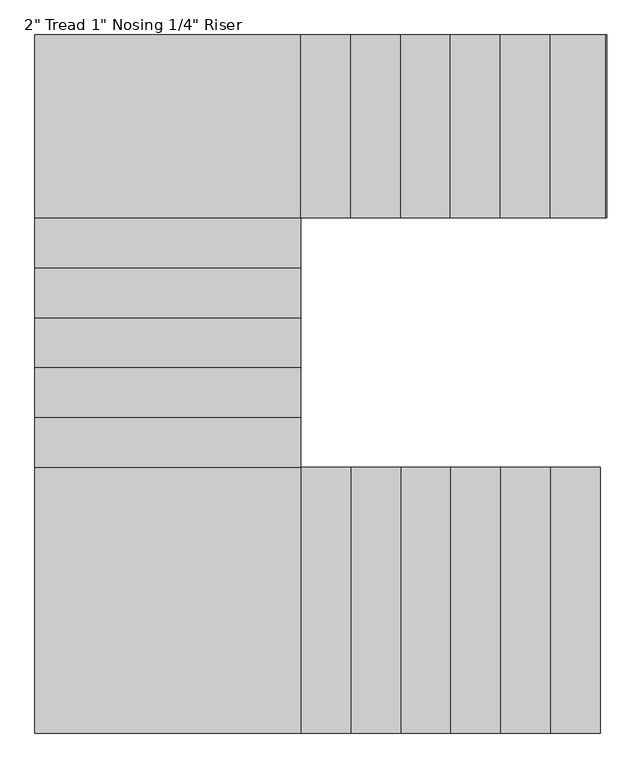
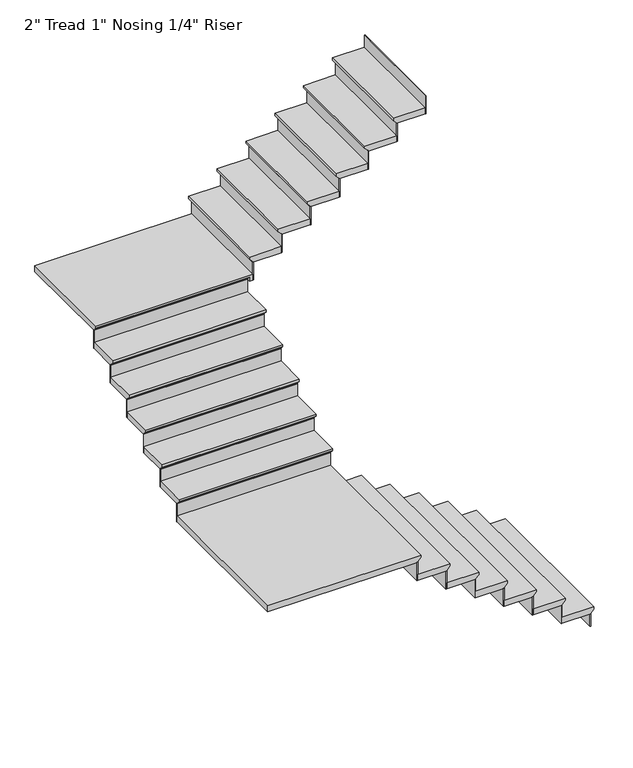
"""IFC4 building model written with IfcOpenShell, lengths in millimetres: stair flight geometry."""

from ifc_helpers import new_model, si_unit, origin, place, context, project, spatial, faceted_brep, source, transform, mapped, element, save


def stair_flight_8a4abe09(model_context):
    return source(origin(), model_context, "Body", "Brep", [
        faceted_brep([(-2515.2117403, -5163.0426559, 3181.35), (-2515.2117403, -5163.0426559, 3200.4), (-2515.2117403, -6382.2426559, 3200.4), (-2515.2117403, -6382.2426559, 3181.35), (-2540.6117403, -5163.0426559, 3155.95), (-2540.6117403, -6382.2426559, 3155.95), (-2769.2117403, -5163.0426559, 3200.4), (-2769.2117403, -6382.2426559, 3200.4), (-2540.6117403, -6382.2426559, 3149.6), (-2769.2117403, -6382.2426559, 3149.6), (-2769.2117403, -5163.0426559, 3149.6), (-2540.6117403, -5163.0426559, 3149.6)], [[[0, 1, 2, 3]], [[4, 0, 3, 5]], [[2, 1, 6, 7]], [[8, 9, 10, 11]], [[2, 7, 9, 8, 5, 3]], [[8, 11, 4, 5]], [[6, 1, 0, 4, 11, 10]], [[7, 6, 10, 9]]]),
        faceted_brep([(-2540.6117403, -5163.0426559, 3149.6), (-2540.6117403, -5163.0426559, 3048.0), (-2546.9617403, -5163.0426559, 3048.0), (-2546.9617403, -5163.0426559, 3149.6), (-2540.6117403, -6382.2426559, 3149.6), (-2546.9617403, -6382.2426559, 3149.6), (-2546.9617403, -6382.2426559, 3048.0), (-2540.6117403, -6382.2426559, 3048.0)], [[[0, 1, 2, 3]], [[4, 5, 6, 7]], [[1, 0, 4, 7]], [[2, 1, 7, 6]], [[3, 2, 6, 5]], [[0, 3, 5, 4]]]),
        faceted_brep([(-2769.2117403, -5163.0426559, 3302.0), (-2769.2117403, -5163.0426559, 3149.6), (-2775.5617403, -5163.0426559, 3149.6), (-2775.5617403, -5163.0426559, 3302.0), (-2769.2117403, -6382.2426559, 3302.0), (-2775.5617403, -6382.2426559, 3302.0), (-2775.5617403, -6382.2426559, 3149.6), (-2769.2117403, -6382.2426559, 3149.6)], [[[0, 1, 2, 3]], [[4, 5, 6, 7]], [[1, 0, 4, 7]], [[2, 1, 7, 6]], [[3, 2, 6, 5]], [[0, 3, 5, 4]]]),
        faceted_brep([(-2743.8117403, -6382.2426559, 3352.8), (-2743.8117403, -5163.0426559, 3352.8), (-2997.8117403, -5163.0426559, 3352.8), (-2997.8117403, -6382.2426559, 3352.8), (-2769.2117403, -6382.2426559, 3302.0), (-2997.8117403, -6382.2426559, 3302.0), (-2997.8117403, -5163.0426559, 3302.0), (-2769.2117403, -5163.0426559, 3302.0), (-2769.2117403, -6382.2426559, 3308.35), (-2743.8117403, -6382.2426559, 3333.75), (-2769.2117403, -5163.0426559, 3308.35), (-2743.8117403, -5163.0426559, 3333.75)], [[[0, 1, 2, 3]], [[4, 5, 6, 7]], [[0, 3, 5, 4, 8, 9]], [[4, 7, 10, 8]], [[2, 1, 11, 10, 7, 6]], [[3, 2, 6, 5]], [[11, 1, 0, 9]], [[10, 11, 9, 8]]]),
        faceted_brep([(-2997.8117403, -5163.0426559, 3454.4), (-2997.8117403, -5163.0426559, 3302.0), (-3004.1617403, -5163.0426559, 3302.0), (-3004.1617403, -5163.0426559, 3454.4), (-2997.8117403, -6382.2426559, 3454.4), (-3004.1617403, -6382.2426559, 3454.4), (-3004.1617403, -6382.2426559, 3302.0), (-2997.8117403, -6382.2426559, 3302.0)], [[[0, 1, 2, 3]], [[4, 5, 6, 7]], [[1, 0, 4, 7]], [[2, 1, 7, 6]], [[3, 2, 6, 5]], [[0, 3, 5, 4]]]),
        faceted_brep([(-2972.4117403, -6382.2426559, 3505.2), (-2972.4117403, -5163.0426559, 3505.2), (-3226.4117403, -5163.0426559, 3505.2), (-3226.4117403, -6382.2426559, 3505.2), (-2997.8117403, -6382.2426559, 3454.4), (-3226.4117403, -6382.2426559, 3454.4), (-3226.4117403, -5163.0426559, 3454.4), (-2997.8117403, -5163.0426559, 3454.4), (-2997.8117403, -6382.2426559, 3460.75), (-2972.4117403, -6382.2426559, 3486.15), (-2997.8117403, -5163.0426559, 3460.75), (-2972.4117403, -5163.0426559, 3486.15)], [[[0, 1, 2, 3]], [[4, 5, 6, 7]], [[0, 3, 5, 4, 8, 9]], [[4, 7, 10, 8]], [[2, 1, 11, 10, 7, 6]], [[3, 2, 6, 5]], [[11, 1, 0, 9]], [[10, 11, 9, 8]]]),
        faceted_brep([(-3226.4117403, -5163.0426559, 3606.8), (-3226.4117403, -5163.0426559, 3454.4), (-3232.7617403, -5163.0426559, 3454.4), (-3232.7617403, -5163.0426559, 3606.8), (-3226.4117403, -6382.2426559, 3606.8), (-3232.7617403, -6382.2426559, 3606.8), (-3232.7617403, -6382.2426559, 3454.4), (-3226.4117403, -6382.2426559, 3454.4)], [[[0, 1, 2, 3]], [[4, 5, 6, 7]], [[1, 0, 4, 7]], [[2, 1, 7, 6]], [[3, 2, 6, 5]], [[0, 3, 5, 4]]]),
        faceted_brep([(-3201.0117403, -6382.2426559, 3657.6), (-3201.0117403, -5163.0426559, 3657.6), (-3455.0117403, -5163.0426559, 3657.6), (-3455.0117403, -6382.2426559, 3657.6), (-3226.4117403, -6382.2426559, 3606.8), (-3455.0117403, -6382.2426559, 3606.8), (-3455.0117403, -5163.0426559, 3606.8), (-3226.4117403, -5163.0426559, 3606.8), (-3226.4117403, -6382.2426559, 3613.15), (-3201.0117403, -6382.2426559, 3638.55), (-3226.4117403, -5163.0426559, 3613.15), (-3201.0117403, -5163.0426559, 3638.55)], [[[0, 1, 2, 3]], [[4, 5, 6, 7]], [[0, 3, 5, 4, 8, 9]], [[4, 7, 10, 8]], [[2, 1, 11, 10, 7, 6]], [[3, 2, 6, 5]], [[11, 1, 0, 9]], [[10, 11, 9, 8]]]),
        faceted_brep([(-3455.0117403, -5163.0426559, 3759.2), (-3455.0117403, -5163.0426559, 3606.8), (-3461.3617403, -5163.0426559, 3606.8), (-3461.3617403, -5163.0426559, 3759.2), (-3455.0117403, -6382.2426559, 3759.2), (-3461.3617403, -6382.2426559, 3759.2), (-3461.3617403, -6382.2426559, 3606.8), (-3455.0117403, -6382.2426559, 3606.8)], [[[0, 1, 2, 3]], [[4, 5, 6, 7]], [[1, 0, 4, 7]], [[2, 1, 7, 6]], [[3, 2, 6, 5]], [[0, 3, 5, 4]]]),
        faceted_brep([(-3429.6117403, -6382.2426559, 3810.0), (-3429.6117403, -5163.0426559, 3810.0), (-3683.6117403, -5163.0426559, 3810.0), (-3683.6117403, -6382.2426559, 3810.0), (-3455.0117403, -6382.2426559, 3759.2), (-3683.6117403, -6382.2426559, 3759.2), (-3683.6117403, -5163.0426559, 3759.2), (-3455.0117403, -5163.0426559, 3759.2), (-3455.0117403, -6382.2426559, 3765.55), (-3429.6117403, -6382.2426559, 3790.95), (-3455.0117403, -5163.0426559, 3765.55), (-3429.6117403, -5163.0426559, 3790.95)], [[[0, 1, 2, 3]], [[4, 5, 6, 7]], [[0, 3, 5, 4, 8, 9]], [[4, 7, 10, 8]], [[2, 1, 11, 10, 7, 6]], [[3, 2, 6, 5]], [[11, 1, 0, 9]], [[10, 11, 9, 8]]]),
        faceted_brep([(-3683.6117403, -5163.0426559, 3911.6), (-3683.6117403, -5163.0426559, 3759.2), (-3689.9617403, -5163.0426559, 3759.2), (-3689.9617403, -5163.0426559, 3911.6), (-3683.6117403, -6382.2426559, 3911.6), (-3689.9617403, -6382.2426559, 3911.6), (-3689.9617403, -6382.2426559, 3759.2), (-3683.6117403, -6382.2426559, 3759.2)], [[[0, 1, 2, 3]], [[4, 5, 6, 7]], [[1, 0, 4, 7]], [[2, 1, 7, 6]], [[3, 2, 6, 5]], [[0, 3, 5, 4]]]),
        faceted_brep([(-3658.2117403, -6382.2426559, 3962.4), (-3658.2117403, -5163.0426559, 3962.4), (-3912.2117403, -5163.0426559, 3962.4), (-3912.2117403, -6382.2426559, 3962.4), (-3683.6117403, -6382.2426559, 3911.6), (-3912.2117403, -6382.2426559, 3911.6), (-3912.2117403, -5163.0426559, 3911.6), (-3683.6117403, -5163.0426559, 3911.6), (-3683.6117403, -6382.2426559, 3917.95), (-3658.2117403, -6382.2426559, 3943.35), (-3683.6117403, -5163.0426559, 3917.95), (-3658.2117403, -5163.0426559, 3943.35)], [[[0, 1, 2, 3]], [[4, 5, 6, 7]], [[0, 3, 5, 4, 8, 9]], [[4, 7, 10, 8]], [[2, 1, 11, 10, 7, 6]], [[3, 2, 6, 5]], [[11, 1, 0, 9]], [[10, 11, 9, 8]]]),
        faceted_brep([(-3912.2117403, -5163.0426559, 4064.0), (-3912.2117403, -5163.0426559, 3911.6), (-3918.5617403, -5163.0426559, 3911.6), (-3918.5617403, -5163.0426559, 4064.0), (-3912.2117403, -6382.2426559, 4064.0), (-3918.5617403, -6382.2426559, 4064.0), (-3918.5617403, -6382.2426559, 3911.6), (-3912.2117403, -6382.2426559, 3911.6)], [[[0, 1, 2, 3]], [[4, 5, 6, 7]], [[1, 0, 4, 7]], [[2, 1, 7, 6]], [[3, 2, 6, 5]], [[0, 3, 5, 4]]]),
        faceted_brep([(-5106.0117403, -5137.6426559, 4114.8), (-5106.0117403, -6382.2426559, 4114.8), (-3886.8117403, -6382.2426559, 4114.8), (-3886.8117403, -5137.6426559, 4114.8), (-5106.0117403, -6382.2426559, 4064.0), (-5106.0117403, -5137.6426559, 4064.0), (-3886.8117403, -5137.6426559, 4064.0), (-3886.8117403, -5163.0426559, 4064.0), (-3912.2117403, -5163.0426559, 4064.0), (-3912.2117403, -6382.2426559, 4064.0), (-3912.2117403, -6382.2426559, 4070.35), (-3886.8117403, -6382.2426559, 4095.75), (-3912.2117403, -5163.0426559, 4070.35), (-3886.8117403, -5163.0426559, 4095.75)], [[[0, 1, 2, 3]], [[4, 5, 6, 7, 8, 9]], [[1, 0, 5, 4]], [[2, 1, 4, 9, 10, 11]], [[9, 8, 12, 10]], [[8, 7, 13, 12]], [[3, 2, 11, 13, 7, 6]], [[0, 3, 6, 5]], [[11, 10, 12, 13]]]),
        faceted_brep([(-3886.8117403, -5137.6426559, 4216.4), (-3886.8117403, -5137.6426559, 4064.0), (-3886.8117403, -5131.2926559, 4064.0), (-3886.8117403, -5131.2926559, 4216.4), (-5106.0117403, -5137.6426559, 4216.4), (-5106.0117403, -5131.2926559, 4216.4), (-5106.0117403, -5131.2926559, 4064.0), (-5106.0117403, -5137.6426559, 4064.0)], [[[0, 1, 2, 3]], [[4, 5, 6, 7]], [[1, 0, 4, 7]], [[2, 1, 7, 6]], [[3, 2, 6, 5]], [[0, 3, 5, 4]]]),
        faceted_brep([(-5106.0117403, -5163.0426559, 4267.2), (-3886.8117403, -5163.0426559, 4267.2), (-3886.8117403, -4909.0426559, 4267.2), (-5106.0117403, -4909.0426559, 4267.2), (-5106.0117403, -5137.6426559, 4216.4), (-5106.0117403, -4909.0426559, 4216.4), (-3886.8117403, -4909.0426559, 4216.4), (-3886.8117403, -5137.6426559, 4216.4), (-5106.0117403, -5137.6426559, 4222.75), (-5106.0117403, -5163.0426559, 4248.15), (-3886.8117403, -5137.6426559, 4222.75), (-3886.8117403, -5163.0426559, 4248.15)], [[[0, 1, 2, 3]], [[4, 5, 6, 7]], [[0, 3, 5, 4, 8, 9]], [[4, 7, 10, 8]], [[2, 1, 11, 10, 7, 6]], [[3, 2, 6, 5]], [[11, 1, 0, 9]], [[10, 11, 9, 8]]]),
        faceted_brep([(-3886.8117403, -4909.0426559, 4368.8), (-3886.8117403, -4909.0426559, 4216.4), (-3886.8117403, -4902.6926559, 4216.4), (-3886.8117403, -4902.6926559, 4368.8), (-5106.0117403, -4909.0426559, 4368.8), (-5106.0117403, -4902.6926559, 4368.8), (-5106.0117403, -4902.6926559, 4216.4), (-5106.0117403, -4909.0426559, 4216.4)], [[[0, 1, 2, 3]], [[4, 5, 6, 7]], [[1, 0, 4, 7]], [[2, 1, 7, 6]], [[3, 2, 6, 5]], [[0, 3, 5, 4]]]),
        faceted_brep([(-5106.0117403, -4934.4426559, 4419.6), (-3886.8117403, -4934.4426559, 4419.6), (-3886.8117403, -4680.4426559, 4419.6), (-5106.0117403, -4680.4426559, 4419.6), (-5106.0117403, -4909.0426559, 4368.8), (-5106.0117403, -4680.4426559, 4368.8), (-3886.8117403, -4680.4426559, 4368.8), (-3886.8117403, -4909.0426559, 4368.8), (-5106.0117403, -4909.0426559, 4375.15), (-5106.0117403, -4934.4426559, 4400.55), (-3886.8117403, -4909.0426559, 4375.15), (-3886.8117403, -4934.4426559, 4400.55)], [[[0, 1, 2, 3]], [[4, 5, 6, 7]], [[0, 3, 5, 4, 8, 9]], [[4, 7, 10, 8]], [[2, 1, 11, 10, 7, 6]], [[3, 2, 6, 5]], [[11, 1, 0, 9]], [[10, 11, 9, 8]]]),
        faceted_brep([(-3886.8117403, -4680.4426559, 4521.2), (-3886.8117403, -4680.4426559, 4368.8), (-3886.8117403, -4674.0926559, 4368.8), (-3886.8117403, -4674.0926559, 4521.2), (-5106.0117403, -4680.4426559, 4521.2), (-5106.0117403, -4674.0926559, 4521.2), (-5106.0117403, -4674.0926559, 4368.8), (-5106.0117403, -4680.4426559, 4368.8)], [[[0, 1, 2, 3]], [[4, 5, 6, 7]], [[1, 0, 4, 7]], [[2, 1, 7, 6]], [[3, 2, 6, 5]], [[0, 3, 5, 4]]]),
        faceted_brep([(-5106.0117403, -4705.8426559, 4572.0), (-3886.8117403, -4705.8426559, 4572.0), (-3886.8117403, -4451.8426559, 4572.0), (-5106.0117403, -4451.8426559, 4572.0), (-5106.0117403, -4680.4426559, 4521.2), (-5106.0117403, -4451.8426559, 4521.2), (-3886.8117403, -4451.8426559, 4521.2), (-3886.8117403, -4680.4426559, 4521.2), (-5106.0117403, -4680.4426559, 4527.55), (-5106.0117403, -4705.8426559, 4552.95), (-3886.8117403, -4680.4426559, 4527.55), (-3886.8117403, -4705.8426559, 4552.95)], [[[0, 1, 2, 3]], [[4, 5, 6, 7]], [[0, 3, 5, 4, 8, 9]], [[4, 7, 10, 8]], [[2, 1, 11, 10, 7, 6]], [[3, 2, 6, 5]], [[11, 1, 0, 9]], [[10, 11, 9, 8]]]),
        faceted_brep([(-3886.8117403, -4451.8426559, 4673.6), (-3886.8117403, -4451.8426559, 4521.2), (-3886.8117403, -4445.4926559, 4521.2), (-3886.8117403, -4445.4926559, 4673.6), (-5106.0117403, -4451.8426559, 4673.6), (-5106.0117403, -4445.4926559, 4673.6), (-5106.0117403, -4445.4926559, 4521.2), (-5106.0117403, -4451.8426559, 4521.2)], [[[0, 1, 2, 3]], [[4, 5, 6, 7]], [[1, 0, 4, 7]], [[2, 1, 7, 6]], [[3, 2, 6, 5]], [[0, 3, 5, 4]]]),
        faceted_brep([(-5106.0117403, -4477.2426559, 4724.4), (-3886.8117403, -4477.2426559, 4724.4), (-3886.8117403, -4223.2426559, 4724.4), (-5106.0117403, -4223.2426559, 4724.4), (-5106.0117403, -4451.8426559, 4673.6), (-5106.0117403, -4223.2426559, 4673.6), (-3886.8117403, -4223.2426559, 4673.6), (-3886.8117403, -4451.8426559, 4673.6), (-5106.0117403, -4451.8426559, 4679.95), (-5106.0117403, -4477.2426559, 4705.35), (-3886.8117403, -4451.8426559, 4679.95), (-3886.8117403, -4477.2426559, 4705.35)], [[[0, 1, 2, 3]], [[4, 5, 6, 7]], [[0, 3, 5, 4, 8, 9]], [[4, 7, 10, 8]], [[2, 1, 11, 10, 7, 6]], [[3, 2, 6, 5]], [[11, 1, 0, 9]], [[10, 11, 9, 8]]]),
        faceted_brep([(-3886.8117403, -4223.2426559, 4826.0), (-3886.8117403, -4223.2426559, 4673.6), (-3886.8117403, -4216.8926559, 4673.6), (-3886.8117403, -4216.8926559, 4826.0), (-5106.0117403, -4223.2426559, 4826.0), (-5106.0117403, -4216.8926559, 4826.0), (-5106.0117403, -4216.8926559, 4673.6), (-5106.0117403, -4223.2426559, 4673.6)], [[[0, 1, 2, 3]], [[4, 5, 6, 7]], [[1, 0, 4, 7]], [[2, 1, 7, 6]], [[3, 2, 6, 5]], [[0, 3, 5, 4]]]),
        faceted_brep([(-5106.0117403, -4248.6426559, 4876.8), (-3886.8117403, -4248.6426559, 4876.8), (-3886.8117403, -3994.6426559, 4876.8), (-5106.0117403, -3994.6426559, 4876.8), (-5106.0117403, -4223.2426559, 4826.0), (-5106.0117403, -3994.6426559, 4826.0), (-3886.8117403, -3994.6426559, 4826.0), (-3886.8117403, -4223.2426559, 4826.0), (-5106.0117403, -4223.2426559, 4832.35), (-5106.0117403, -4248.6426559, 4857.75), (-3886.8117403, -4223.2426559, 4832.35), (-3886.8117403, -4248.6426559, 4857.75)], [[[0, 1, 2, 3]], [[4, 5, 6, 7]], [[0, 3, 5, 4, 8, 9]], [[4, 7, 10, 8]], [[2, 1, 11, 10, 7, 6]], [[3, 2, 6, 5]], [[11, 1, 0, 9]], [[10, 11, 9, 8]]]),
        faceted_brep([(-3886.8117403, -3994.6426559, 4978.4), (-3886.8117403, -3994.6426559, 4826.0), (-3886.8117403, -3988.2926559, 4826.0), (-3886.8117403, -3988.2926559, 4978.4), (-5106.0117403, -3994.6426559, 4978.4), (-5106.0117403, -3988.2926559, 4978.4), (-5106.0117403, -3988.2926559, 4826.0), (-5106.0117403, -3994.6426559, 4826.0)], [[[0, 1, 2, 3]], [[4, 5, 6, 7]], [[1, 0, 4, 7]], [[2, 1, 7, 6]], [[3, 2, 6, 5]], [[0, 3, 5, 4]]]),
        faceted_brep([(-3861.4117403, -3181.8426559, 5029.2), (-5106.0117403, -3181.8426559, 5029.2), (-5106.0117403, -4020.0426559, 5029.2), (-3861.4117403, -4020.0426559, 5029.2), (-5106.0117403, -3181.8426559, 4978.4), (-3861.4117403, -3181.8426559, 4978.4), (-3861.4117403, -4020.0426559, 4978.4), (-3886.8117403, -4020.0426559, 4978.4), (-3886.8117403, -3994.6426559, 4978.4), (-5106.0117403, -3994.6426559, 4978.4), (-5106.0117403, -3994.6426559, 4984.75), (-5106.0117403, -4020.0426559, 5010.15), (-3886.8117403, -3994.6426559, 4984.75), (-3886.8117403, -4020.0426559, 5010.15)], [[[0, 1, 2, 3]], [[4, 5, 6, 7, 8, 9]], [[1, 0, 5, 4]], [[2, 1, 4, 9, 10, 11]], [[9, 8, 12, 10]], [[8, 7, 13, 12]], [[3, 2, 11, 13, 7, 6]], [[0, 3, 6, 5]], [[11, 10, 12, 13]]]),
        faceted_brep([(-3861.4117403, -4020.0426559, 5130.8), (-3861.4117403, -4020.0426559, 4978.4), (-3855.0617403, -4020.0426559, 4978.4), (-3855.0617403, -4020.0426559, 5130.8), (-3861.4117403, -3181.8426559, 5130.8), (-3855.0617403, -3181.8426559, 5130.8), (-3855.0617403, -3181.8426559, 4978.4), (-3861.4117403, -3181.8426559, 4978.4)], [[[0, 1, 2, 3]], [[4, 5, 6, 7]], [[1, 0, 4, 7]], [[2, 1, 7, 6]], [[3, 2, 6, 5]], [[0, 3, 5, 4]]]),
        faceted_brep([(-3886.8117403, -3181.8426559, 5181.6), (-3886.8117403, -4020.0426559, 5181.6), (-3632.8117403, -4020.0426559, 5181.6), (-3632.8117403, -3181.8426559, 5181.6), (-3861.4117403, -3181.8426559, 5130.8), (-3632.8117403, -3181.8426559, 5130.8), (-3632.8117403, -4020.0426559, 5130.8), (-3861.4117403, -4020.0426559, 5130.8), (-3861.4117403, -3181.8426559, 5137.15), (-3886.8117403, -3181.8426559, 5162.55), (-3861.4117403, -4020.0426559, 5137.15), (-3886.8117403, -4020.0426559, 5162.55)], [[[0, 1, 2, 3]], [[4, 5, 6, 7]], [[0, 3, 5, 4, 8, 9]], [[4, 7, 10, 8]], [[2, 1, 11, 10, 7, 6]], [[3, 2, 6, 5]], [[11, 1, 0, 9]], [[10, 11, 9, 8]]]),
        faceted_brep([(-3632.8117403, -4020.0426559, 5283.2), (-3632.8117403, -4020.0426559, 5130.8), (-3626.4617403, -4020.0426559, 5130.8), (-3626.4617403, -4020.0426559, 5283.2), (-3632.8117403, -3181.8426559, 5283.2), (-3626.4617403, -3181.8426559, 5283.2), (-3626.4617403, -3181.8426559, 5130.8), (-3632.8117403, -3181.8426559, 5130.8)], [[[0, 1, 2, 3]], [[4, 5, 6, 7]], [[1, 0, 4, 7]], [[2, 1, 7, 6]], [[3, 2, 6, 5]], [[0, 3, 5, 4]]]),
        faceted_brep([(-3658.2117403, -3181.8426559, 5334.0), (-3658.2117403, -4020.0426559, 5334.0), (-3404.2117403, -4020.0426559, 5334.0), (-3404.2117403, -3181.8426559, 5334.0), (-3632.8117403, -3181.8426559, 5283.2), (-3404.2117403, -3181.8426559, 5283.2), (-3404.2117403, -4020.0426559, 5283.2), (-3632.8117403, -4020.0426559, 5283.2), (-3632.8117403, -3181.8426559, 5289.55), (-3658.2117403, -3181.8426559, 5314.95), (-3632.8117403, -4020.0426559, 5289.55), (-3658.2117403, -4020.0426559, 5314.95)], [[[0, 1, 2, 3]], [[4, 5, 6, 7]], [[0, 3, 5, 4, 8, 9]], [[4, 7, 10, 8]], [[2, 1, 11, 10, 7, 6]], [[3, 2, 6, 5]], [[11, 1, 0, 9]], [[10, 11, 9, 8]]]),
        faceted_brep([(-3404.2117403, -4020.0426559, 5435.6), (-3404.2117403, -4020.0426559, 5283.2), (-3397.8617403, -4020.0426559, 5283.2), (-3397.8617403, -4020.0426559, 5435.6), (-3404.2117403, -3181.8426559, 5435.6), (-3397.8617403, -3181.8426559, 5435.6), (-3397.8617403, -3181.8426559, 5283.2), (-3404.2117403, -3181.8426559, 5283.2)], [[[0, 1, 2, 3]], [[4, 5, 6, 7]], [[1, 0, 4, 7]], [[2, 1, 7, 6]], [[3, 2, 6, 5]], [[0, 3, 5, 4]]]),
        faceted_brep([(-3429.6117403, -3181.8426559, 5486.4), (-3429.6117403, -4020.0426559, 5486.4), (-3175.6117403, -4020.0426559, 5486.4), (-3175.6117403, -3181.8426559, 5486.4), (-3404.2117403, -3181.8426559, 5435.6), (-3175.6117403, -3181.8426559, 5435.6), (-3175.6117403, -4020.0426559, 5435.6), (-3404.2117403, -4020.0426559, 5435.6), (-3404.2117403, -3181.8426559, 5441.95), (-3429.6117403, -3181.8426559, 5467.35), (-3404.2117403, -4020.0426559, 5441.95), (-3429.6117403, -4020.0426559, 5467.35)], [[[0, 1, 2, 3]], [[4, 5, 6, 7]], [[0, 3, 5, 4, 8, 9]], [[4, 7, 10, 8]], [[2, 1, 11, 10, 7, 6]], [[3, 2, 6, 5]], [[11, 1, 0, 9]], [[10, 11, 9, 8]]]),
        faceted_brep([(-3175.6117403, -4020.0426559, 5588.0), (-3175.6117403, -4020.0426559, 5435.6), (-3169.2617403, -4020.0426559, 5435.6), (-3169.2617403, -4020.0426559, 5588.0), (-3175.6117403, -3181.8426559, 5588.0), (-3169.2617403, -3181.8426559, 5588.0), (-3169.2617403, -3181.8426559, 5435.6), (-3175.6117403, -3181.8426559, 5435.6)], [[[0, 1, 2, 3]], [[4, 5, 6, 7]], [[1, 0, 4, 7]], [[2, 1, 7, 6]], [[3, 2, 6, 5]], [[0, 3, 5, 4]]]),
        faceted_brep([(-3201.0117403, -3181.8426559, 5638.8), (-3201.0117403, -4020.0426559, 5638.8), (-2947.0117403, -4020.0426559, 5638.8), (-2947.0117403, -3181.8426559, 5638.8), (-3175.6117403, -3181.8426559, 5588.0), (-2947.0117403, -3181.8426559, 5588.0), (-2947.0117403, -4020.0426559, 5588.0), (-3175.6117403, -4020.0426559, 5588.0), (-3175.6117403, -3181.8426559, 5594.35), (-3201.0117403, -3181.8426559, 5619.75), (-3175.6117403, -4020.0426559, 5594.35), (-3201.0117403, -4020.0426559, 5619.75)], [[[0, 1, 2, 3]], [[4, 5, 6, 7]], [[0, 3, 5, 4, 8, 9]], [[4, 7, 10, 8]], [[2, 1, 11, 10, 7, 6]], [[3, 2, 6, 5]], [[11, 1, 0, 9]], [[10, 11, 9, 8]]]),
        faceted_brep([(-2947.0117403, -4020.0426559, 5740.4), (-2947.0117403, -4020.0426559, 5588.0), (-2940.6617403, -4020.0426559, 5588.0), (-2940.6617403, -4020.0426559, 5740.4), (-2947.0117403, -3181.8426559, 5740.4), (-2940.6617403, -3181.8426559, 5740.4), (-2940.6617403, -3181.8426559, 5588.0), (-2947.0117403, -3181.8426559, 5588.0)], [[[0, 1, 2, 3]], [[4, 5, 6, 7]], [[1, 0, 4, 7]], [[2, 1, 7, 6]], [[3, 2, 6, 5]], [[0, 3, 5, 4]]]),
        faceted_brep([(-2972.4117403, -3181.8426559, 5791.2), (-2972.4117403, -4020.0426559, 5791.2), (-2718.4117403, -4020.0426559, 5791.2), (-2718.4117403, -3181.8426559, 5791.2), (-2947.0117403, -3181.8426559, 5740.4), (-2718.4117403, -3181.8426559, 5740.4), (-2718.4117403, -4020.0426559, 5740.4), (-2947.0117403, -4020.0426559, 5740.4), (-2947.0117403, -3181.8426559, 5746.75), (-2972.4117403, -3181.8426559, 5772.15), (-2947.0117403, -4020.0426559, 5746.75), (-2972.4117403, -4020.0426559, 5772.15)], [[[0, 1, 2, 3]], [[4, 5, 6, 7]], [[0, 3, 5, 4, 8, 9]], [[4, 7, 10, 8]], [[2, 1, 11, 10, 7, 6]], [[3, 2, 6, 5]], [[11, 1, 0, 9]], [[10, 11, 9, 8]]]),
        faceted_brep([(-2718.4117403, -4020.0426559, 5892.8), (-2718.4117403, -4020.0426559, 5740.4), (-2712.0617403, -4020.0426559, 5740.4), (-2712.0617403, -4020.0426559, 5892.8), (-2718.4117403, -3181.8426559, 5892.8), (-2712.0617403, -3181.8426559, 5892.8), (-2712.0617403, -3181.8426559, 5740.4), (-2718.4117403, -3181.8426559, 5740.4)], [[[0, 1, 2, 3]], [[4, 5, 6, 7]], [[1, 0, 4, 7]], [[2, 1, 7, 6]], [[3, 2, 6, 5]], [[0, 3, 5, 4]]]),
        faceted_brep([(-2489.8117403, -4020.0426559, 6045.2), (-2489.8117403, -4020.0426559, 5892.8), (-2483.4617403, -4020.0426559, 5892.8), (-2483.4617403, -4020.0426559, 6045.2), (-2489.8117403, -3181.8426559, 6045.2), (-2483.4617403, -3181.8426559, 6045.2), (-2483.4617403, -3181.8426559, 5892.8), (-2489.8117403, -3181.8426559, 5892.8)], [[[0, 1, 2, 3]], [[4, 5, 6, 7]], [[1, 0, 4, 7]], [[2, 1, 7, 6]], [[3, 2, 6, 5]], [[0, 3, 5, 4]]]),
        faceted_brep([(-2743.8117403, -3181.8426559, 5943.6), (-2743.8117403, -4020.0426559, 5943.6), (-2489.8117403, -4020.0426559, 5943.6), (-2489.8117403, -3181.8426559, 5943.6), (-2718.4117403, -3181.8426559, 5892.8), (-2489.8117403, -3181.8426559, 5892.8), (-2489.8117403, -4020.0426559, 5892.8), (-2718.4117403, -4020.0426559, 5892.8), (-2718.4117403, -3181.8426559, 5899.15), (-2743.8117403, -3181.8426559, 5924.55), (-2718.4117403, -4020.0426559, 5899.15), (-2743.8117403, -4020.0426559, 5924.55)], [[[0, 1, 2, 3]], [[4, 5, 6, 7]], [[0, 3, 5, 4, 8, 9]], [[4, 7, 10, 8]], [[2, 1, 11, 10, 7, 6]], [[3, 2, 6, 5]], [[11, 1, 0, 9]], [[10, 11, 9, 8]]]),
    ])


if __name__ == "__main__":
    model = new_model("IFC4")
    model_context = context("Model", 3, world=origin())
    ifc_project = project(units=[si_unit("LENGTHUNIT", "METRE", prefix="MILLI")], contexts=[model_context])
    site = spatial("IfcSite", under=ifc_project)
    building = spatial("IfcBuilding", under=site)
    placement = place(None, origin())
    stair_flight_shape = stair_flight_8a4abe09(model_context)
    element("IfcStairFlight", 1, ObjectType="2\" Tread 1\" Nosing 1/4\" Riser", at=placement, inside=building, context=model_context, shape_type="MappedRepresentation", body=[
        mapped(stair_flight_shape, transform((0.0, 0.0, 0.0), x_axis=(1.0, 0.0, 0.0), y_axis=(0.0, 1.0, 0.0), z_axis=(0.0, 0.0, 1.0))),
    ])
    save(model, "model.ifc")

# Revit data of these elements
# Element 1 (IfcStairFlight, "2\" Tread 1\" Nosing 1/4\" Riser")
#   Materials on its faces: "Wood Planks"
# Materials
#   "Wood Planks": class "Wood", colour RGB 193 160 115, transparency 0, Description = "Physical material.", Cost = 0
